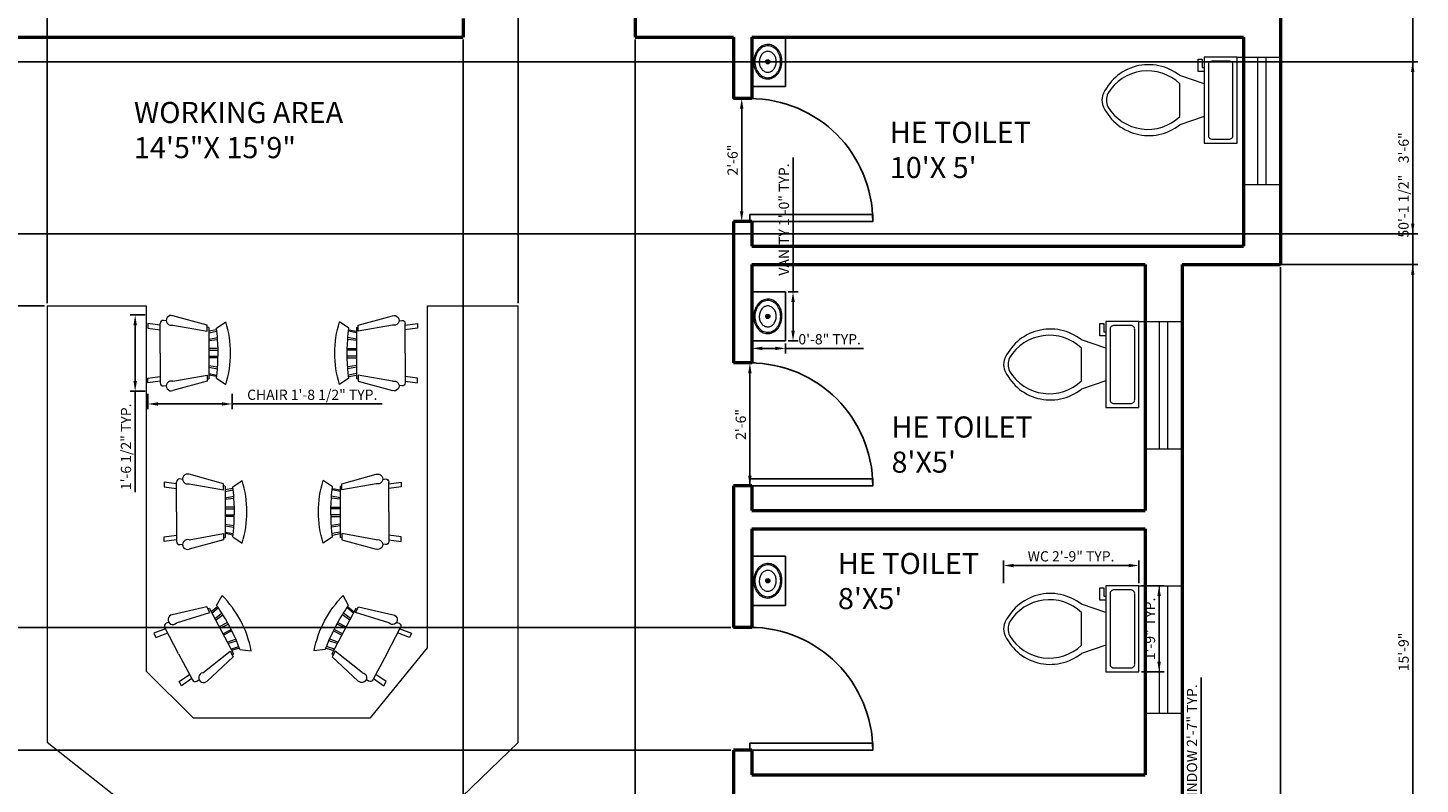
# Model space of a CAD drawing. Units: inches. Extents: x -4852 to -4300, y 4342 to 5059.
# Tile 3 of 4: x -4640 to -4300, y 4580 to 4764. Entities that reach past the tile are written whole.
import ezdxf

# ---------------------------------------------------------------- set-up
doc = ezdxf.new("R2010")
doc.units = ezdxf.units.IN
for name, color, linetype, lineweight in [('A-ANNO-DIMS', 2, 'Continuous', 18), ('A-AREA-IDEN', 7, 'Continuous', 18), ('A-DOOR', 4, 'Continuous', 25), ('A-FLOR-CASE', 9, 'Continuous', 25), ('A-FLOR-FIXT', 9, 'Continuous', 18), ('A-FURN', 8, 'Continuous', 18), ('A-GLAZ', 4, 'Continuous', 18), ('A-WALL', 7, 'Continuous', 50)]:
    doc.layers.add(name, color=color, linetype=linetype, lineweight=lineweight)
doc.styles.get("Standard").update_dxf_attribs({"font": 'arial.ttf'})
doc.dimstyles.new('ISO-25', dxfattribs={"dimtxt": 2.5, "dimasz": 2.5, "dimexe": 1.25, "dimexo": 0.625, "dimtad": 1, "dimdec": 0, "dimlunit": 3, "dimtxsty": 'Standard', "dimcen": 2.5, "dimadec": 0, "dimazin": 0, "dimtfac": 1, "dimtdec": 0, "dimtmove": 0, "dimatfit": 3, "dimfxl": 1, "dimarcsym": 0})

# ---------------------------------------------------------------- blocks, each defined once
blk = doc.blocks.new('*U2')
for p, q in [((0, 0), (0, -100)), ((750, 0), (750, -100))]:
    blk.add_line(p, q)
blk.add_lwpolyline([(0, 0), (0, 750), (43.75, 750), (43.75, 0)], close=True)
blk.add_arc((0, 0), 750, 0, 90)
blk = doc.blocks.new('Toilet - top')
for p, q in [((9.5, -6), (9.5, -2)), ((-10, -8.5), (-8, -8.5)), ((-10, -9.5), (-10, -8.5)), ((-7, -9.5), (-10, -9.5)), ((-8, -8.5), (-8, -8)), ((-7, -8), (-7, -9.5)), ((-4, -8), (-6, -14)), ((4, -8), (6, -14)), ((4, -14), (-4, -14))]:
    blk.add_line(p, q)
blk.add_lwpolyline([(10.5, -8), (10.5, 0), (-10.5, 0), (-10.5, -8)], close=True)
for points in [[(-9.5, -2), (-9.5, -6)], [(8.5, -1), (-8.5, -1)], [(-8.5, -7), (8.5, -7)]]:
    blk.add_lwpolyline(points)
for centre, radius, start, end in [((-8.62, -1.88), 0.884, 81.8699, 188.1301), ((8.62, -1.88), 0.884, 351.8699, 98.1301), ((-8.62, -6.12), 0.884, 171.8699, 278.1301), ((8.62, -6.12), 0.884, 261.8699, 8.1301), ((3.52, -21.58), 12.17, 141.4691, 247.9714), ((4.2, -21.82), 11.33, 136.3677, 238.9468), ((-3.52, -21.58), 12.17, 292.0284, 38.5307), ((-4.2, -21.82), 11.33, 301.053, 43.6321), ((0, -27.88), 4, 245.7318, 294.2682), ((0, -29), 4, 254.8605, 285.1395)]:
    blk.add_arc(centre, radius, start, end)
blk = doc.blocks.new('Sink - Oval top')
for p, q in [((-1, 0), (1, 0)), ((0, 1), (0, -1))]:
    blk.add_line(p, q)
for points in [[(-12.23, 0.39, 0.117634), (-11.46, -3.36, 0.104469), (-8.88, -6.8, 0.090016), (-5.08, -9.07, 0.08192), (-0.32, -10.02, 0.08192), (4.49, -9.38, 0.090016), (8.42, -7.36, 0.104469), (11.22, -4.09, 0.117634), (12.23, -0.39, 0.117634), (11.46, 3.36, 0.104469), (8.88, 6.8, 0.090016), (5.08, 9.07, 0.08192), (0.32, 10.02, 0.08192), (-4.49, 9.38, 0.090016), (-8.42, 7.36, 0.104469), (-11.22, 4.09, 0.117634)], [(-11.29, 0.16, 0.118622), (-10.52, -3.25, 0.104678), (-8.07, -6.36, 0.089562), (-4.54, -8.37, 0.081185), (-0.13, -9.15, 0.081185), (4.3, -8.49, 0.089562), (7.89, -6.58, 0.104678), (10.42, -3.55, 0.118622), (11.29, -0.16, 0.118622), (10.52, 3.25, 0.104678), (8.07, 6.36, 0.089562), (4.54, 8.37, 0.081185), (0.13, 9.15, 0.081185), (-4.3, 8.49, 0.089562), (-7.89, 6.58, 0.104678), (-10.42, 3.55, 0.118622)], [(-7.42, 0.08, 0.118283), (-6.91, -2.17, 0.104607), (-5.29, -4.21, 0.089718), (-2.97, -5.53, 0.081436), (-0.07, -6.04, 0.081436), (2.84, -5.59, 0.089718), (5.2, -4.33, 0.104607), (6.86, -2.32, 0.118283), (7.42, -0.08, 0.118283), (6.91, 2.17, 0.104607), (5.29, 4.21, 0.089718), (2.97, 5.53, 0.081436), (0.07, 6.04, 0.081436), (-2.84, 5.59, 0.089718), (-5.2, 4.33, 0.104607), (-6.86, 2.32, 0.118283)]]:
    blk.add_lwpolyline(points, format="xyb", close=True)
for radius in [1.5, 1]:
    blk.add_circle((0, 0), radius)
blk = doc.blocks.new('Chair - Rocking')
for p, q in [((-8, -4.5), (-10, -1.5)), ((-6.5, -7), (-7.02225, -4.43)), ((-4.5, -7), (-4.96674, -4.19951)), ((-4, -7), (-4.40532, -4.16272)), ((-1.5, -4.05012), (-1.5, -7)), ((-1, -7), (-1, -4.05012)), ((1, -7), (1, -4.04655)), ((1.5, -4.05012), (1.5, -7)), ((4, -7), (4.40187, -4.18694)), ((4.5, -7), (4.96761, -4.19437)), ((6.5, -7), (7, -4.4057)), ((8, -4.5), (10, -1.5)), ((-9, -7.5), (-12, -18.49999)), ((-7, -7.5), (-9, -7.5)), ((-9, -18.49999), (-7, -7.5)), ((-8.23428, -6.99939), (-8.3093, -7.47958)), ((-8.23041, -7), (8.23915, -7)), ((-7.5, -4.5), (-7, -7)), ((7.5, -4.5), (7, -7)), ((7, -7.5), (9, -7.5)), ((9, -18.49999), (7, -7.5)), ((8.31071, -7.48854), (8.23449, -7.00073)), ((9, -7.5), (12, -18.49999)), ((-10.36644, -20.64523), (-10.5, -21.49999)), ((10.5, -21.49999), (10.3575, -20.58798)), ((-9, -22.49999), (-9.5, -26.49999)), ((0, -22.49999), (-9.5, -22.49999)), ((-9.5, -26.49999), (-8, -26.49999)), ((-8, -26.49999), (-7.5, -22.49999)), ((0, -22.49999), (9.5, -22.49999)), ((8, -26.49999), (7.5, -22.49999)), ((9.5, -26.49999), (8, -26.49999)), ((9, -22.49999), (9.5, -26.49999))]:
    blk.add_line(p, q)
for centre, radius, start, end in [((0, -34.08333), 34.08333, 72.93847, 107.0615), ((0, -68.25004), 64.25, 93.92211, 97.15267), ((0, -68.25004), 64.25, 82.84733, 93.92211), ((-10.5, -18.99999), 1.58114, 161.5651, 18.43495), ((-9.5, -21.49999), 1, 180, 270), ((10.5, -18.99999), 1.58114, 161.5651, 18.43495), ((9.5, -21.49999), 1, 270, 0)]:
    blk.add_arc(centre, radius, start, end)
blk = doc.blocks.new('*D12')
at = {"layer": 'A-ANNO-DIMS', "color": 0, "lineweight": -2, "transparency": 16777216}
for p, q in [((-4466.77, 4682.38), (-4462.15, 4682.38)), ((-4463.4, 4679.88), (-4463.4, 4654.88)), ((-4464.52, 4652.38), (-4462.15, 4652.38))]:
    blk.add_line(p, q, dxfattribs=at)
at = {"layer": 'A-ANNO-DIMS', "color": 0, "transparency": 16777216}
for points in [[(-4463.82, 4679.88), (-4462.98, 4679.88), (-4463.4, 4682.38)], [(-4463.82, 4654.88), (-4462.98, 4654.88), (-4463.4, 4652.38)]]:
    blk.add_solid(points, dxfattribs=at)
at = {"layer": 'Defpoints', "color": 0, "transparency": 16777216}
for p in [(-4467.4, 4682.38), (-4465.15, 4652.38), (-4463.4, 4652.38)]:
    blk.add_point(p, dxfattribs=at)
at = {"layer": 'A-ANNO-DIMS', "color": 0, "transparency": 16777216, "insert": (-4465.3, 4667.38), "char_height": 2.5, "attachment_point": 5, "rotation": 90}
blk.add_mtext('2\'-6"', dxfattribs=at)
blk = doc.blocks.new('*D13')
at = {"layer": 'A-ANNO-DIMS', "color": 0, "lineweight": -2, "transparency": 16777216}
for p, q in [((-4466.77, 4746.88), (-4464.15, 4746.88)), ((-4465.4, 4744.38), (-4465.4, 4719.38)), ((-4466.02, 4716.88), (-4466.65, 4716.88))]:
    blk.add_line(p, q, dxfattribs=at)
at = {"layer": 'A-ANNO-DIMS', "color": 0, "transparency": 16777216}
for points in [[(-4465.82, 4744.38), (-4464.98, 4744.38), (-4465.4, 4746.88)], [(-4465.82, 4719.38), (-4464.98, 4719.38), (-4465.4, 4716.88)]]:
    blk.add_solid(points, dxfattribs=at)
at = {"layer": 'Defpoints', "color": 0, "transparency": 16777216}
for p in [(-4467.4, 4746.88), (-4465.4, 4716.88), (-4465.4, 4716.88)]:
    blk.add_point(p, dxfattribs=at)
at = {"layer": 'A-ANNO-DIMS', "color": 0, "transparency": 16777216, "insert": (-4467.3, 4731.88), "char_height": 2.5, "attachment_point": 5, "rotation": 90}
blk.add_mtext('2\'-6"', dxfattribs=at)
blk = doc.blocks.new('VANITY-COMPACT')
for p, q in [((8.23, 12.02), (0, 12.02)), ((8.23, 0), (8.23, 12.02)), ((0, 0), (8.23, 0))]:
    blk.add_line(p, q)
blk = doc.blocks.new('WIN-RESTROOM')
for p, q in [((0, 31.05), (10.57, 31.05)), ((5.07, 0), (5.07, 31.05)), ((7.07, 0), (7.07, 31.05)), ((1.57, 0), (10.57, 0))]:
    blk.add_line(p, q)
blk = doc.blocks.new('*D23')
at = {"layer": 'A-ANNO-DIMS', "color": 0, "lineweight": -2, "transparency": 16777216}
for p, q in [((-4610.37, 4674.84), (-4610.37, 4671.12)), ((-4589.8, 4674.84), (-4589.8, 4671.12)), ((-4607.87, 4672.37), (-4592.3, 4672.37)), ((-4589.8, 4672.37), (-4553.17, 4672.37))]:
    blk.add_line(p, q, dxfattribs=at)
at = {"layer": 'A-ANNO-DIMS', "color": 0, "transparency": 16777216}
for points in [[(-4607.87, 4672.79), (-4607.87, 4671.96), (-4610.37, 4672.37)], [(-4592.3, 4672.79), (-4592.3, 4671.96), (-4589.8, 4672.37)]]:
    blk.add_solid(points, dxfattribs=at)
at = {"layer": 'Defpoints', "color": 0, "transparency": 16777216}
for p in [(-4610.37, 4675.46), (-4589.8, 4675.46), (-4589.8, 4672.37)]:
    blk.add_point(p, dxfattribs=at)
at = {"layer": 'A-ANNO-DIMS', "color": 0, "transparency": 16777216, "insert": (-4570.23, 4674.29), "char_height": 2.5, "attachment_point": 5}
blk.add_mtext('CHAIR 1\'-8 1/2" TYP.', dxfattribs=at)
blk = doc.blocks.new('*D24')
at = {"layer": 'A-ANNO-DIMS', "color": 0, "lineweight": -2, "transparency": 16777216}
for p, q in [((-4611, 4694.08), (-4614.71, 4694.08)), ((-4613.46, 4691.58), (-4613.46, 4677.96)), ((-4611, 4675.46), (-4614.71, 4675.46)), ((-4613.46, 4675.46), (-4613.46, 4650.88))]:
    blk.add_line(p, q, dxfattribs=at)
at = {"layer": 'A-ANNO-DIMS', "color": 0, "transparency": 16777216}
for points in [[(-4613.88, 4691.58), (-4613.04, 4691.58), (-4613.46, 4694.08)], [(-4613.88, 4677.96), (-4613.04, 4677.96), (-4613.46, 4675.46)]]:
    blk.add_solid(points, dxfattribs=at)
at = {"layer": 'Defpoints', "color": 0, "transparency": 16777216}
for p in [(-4610.37, 4694.08), (-4613.46, 4675.46), (-4610.37, 4675.46)]:
    blk.add_point(p, dxfattribs=at)
at = {"layer": 'A-ANNO-DIMS', "color": 0, "transparency": 16777216, "insert": (-4615.38, 4661.92), "char_height": 2.5, "attachment_point": 5, "rotation": 90}
blk.add_mtext('1\'-6 1/2" TYP.', dxfattribs=at)
blk = doc.blocks.new('*D27')
at = {"layer": 'A-ANNO-DIMS', "color": 0, "lineweight": -2, "transparency": 16777216}
for p, q in [((-4401.51, 4628.63), (-4401.51, 4634.21)), ((-4399.01, 4632.96), (-4370.97, 4632.96)), ((-4368.47, 4628.63), (-4368.47, 4634.21))]:
    blk.add_line(p, q, dxfattribs=at)
at = {"layer": 'A-ANNO-DIMS', "color": 0, "transparency": 16777216}
for points in [[(-4399.01, 4633.38), (-4399.01, 4632.54), (-4401.51, 4632.96)], [(-4370.97, 4633.38), (-4370.97, 4632.54), (-4368.47, 4632.96)]]:
    blk.add_solid(points, dxfattribs=at)
at = {"layer": 'Defpoints', "color": 0, "transparency": 16777216}
for p in [(-4368.47, 4632.96), (-4401.51, 4628), (-4368.47, 4628)]:
    blk.add_point(p, dxfattribs=at)
at = {"layer": 'A-ANNO-DIMS', "color": 0, "transparency": 16777216, "insert": (-4384.99, 4634.88), "char_height": 2.5, "attachment_point": 5}
blk.add_mtext('WC 2\'-9" TYP.', dxfattribs=at)
blk = doc.blocks.new('*D28')
at = {"layer": 'A-ANNO-DIMS', "color": 0, "lineweight": -2, "transparency": 16777216}
for p, q in [((-4367.84, 4628), (-4362.26, 4628)), ((-4363.51, 4625.5), (-4363.51, 4609.5)), ((-4367.84, 4607), (-4362.26, 4607))]:
    blk.add_line(p, q, dxfattribs=at)
at = {"layer": 'A-ANNO-DIMS', "color": 0, "transparency": 16777216}
for points in [[(-4363.93, 4625.5), (-4363.09, 4625.5), (-4363.51, 4628)], [(-4363.93, 4609.5), (-4363.09, 4609.5), (-4363.51, 4607)]]:
    blk.add_solid(points, dxfattribs=at)
at = {"layer": 'Defpoints', "color": 0, "transparency": 16777216}
for p in [(-4368.47, 4628), (-4368.47, 4607), (-4363.51, 4607)]:
    blk.add_point(p, dxfattribs=at)
at = {"layer": 'A-ANNO-DIMS', "color": 0, "transparency": 16777216, "insert": (-4365.41, 4617.5), "char_height": 2.5, "attachment_point": 5, "rotation": 90}
blk.add_mtext('1\'-9" TYP.', dxfattribs=at)
blk = doc.blocks.new('*D33')
at = {"layer": 'A-ANNO-DIMS', "color": 0, "lineweight": -2, "transparency": 16777216}
for p, q in [((-4452.87, 4699.76), (-4452.87, 4732.47)), ((-4454.04, 4699.76), (-4451.62, 4699.76)), ((-4452.87, 4690.24), (-4452.87, 4697.26)), ((-4454.04, 4687.74), (-4451.62, 4687.74))]:
    blk.add_line(p, q, dxfattribs=at)
at = {"layer": 'A-ANNO-DIMS', "color": 0, "transparency": 16777216}
for points in [[(-4453.28, 4697.26), (-4452.45, 4697.26), (-4452.87, 4699.76)], [(-4453.28, 4690.24), (-4452.45, 4690.24), (-4452.87, 4687.74)]]:
    blk.add_solid(points, dxfattribs=at)
at = {"layer": 'Defpoints', "color": 0, "transparency": 16777216}
for p in [(-4454.67, 4699.76), (-4452.87, 4699.76), (-4454.67, 4687.74)]:
    blk.add_point(p, dxfattribs=at)
at = {"layer": 'A-ANNO-DIMS', "color": 0, "transparency": 16777216, "insert": (-4454.77, 4717.37), "char_height": 2.5, "attachment_point": 5, "rotation": 90}
blk.add_mtext('VANITY 1\'-0" TYP.', dxfattribs=at)
blk = doc.blocks.new('*D34')
at = {"layer": 'A-ANNO-DIMS', "color": 0, "lineweight": -2, "transparency": 16777216}
for p, q in [((-4462.9, 4687.12), (-4462.9, 4684.69)), ((-4454.67, 4687.12), (-4454.67, 4684.69)), ((-4460.4, 4685.94), (-4457.17, 4685.94)), ((-4454.67, 4685.94), (-4435.68, 4685.94))]:
    blk.add_line(p, q, dxfattribs=at)
at = {"layer": 'A-ANNO-DIMS', "color": 0, "transparency": 16777216}
for points in [[(-4460.4, 4686.35), (-4460.4, 4685.52), (-4462.9, 4685.94)], [(-4457.17, 4686.35), (-4457.17, 4685.52), (-4454.67, 4685.94)]]:
    blk.add_solid(points, dxfattribs=at)
at = {"layer": 'Defpoints', "color": 0, "transparency": 16777216}
for p in [(-4462.9, 4687.74), (-4454.67, 4687.74), (-4454.67, 4685.94)]:
    blk.add_point(p, dxfattribs=at)
at = {"layer": 'A-ANNO-DIMS', "color": 0, "transparency": 16777216, "insert": (-4443.93, 4687.84), "char_height": 2.5, "attachment_point": 5}
blk.add_mtext('0\'-8" TYP.', dxfattribs=at)
blk = doc.blocks.new('*D35')
at = {"layer": 'A-ANNO-DIMS', "color": 0, "lineweight": -2, "transparency": 16777216}
for p, q in [((-4353.24, 4563.5), (-4353.24, 4605.68)), ((-4357.27, 4563.5), (-4351.99, 4563.5)), ((-4353.24, 4534.95), (-4353.24, 4561)), ((-4357.27, 4532.45), (-4351.99, 4532.45))]:
    blk.add_line(p, q, dxfattribs=at)
at = {"layer": 'A-ANNO-DIMS', "color": 0, "transparency": 16777216}
for points in [[(-4353.66, 4561), (-4352.83, 4561), (-4353.24, 4563.5)], [(-4353.66, 4534.95), (-4352.83, 4534.95), (-4353.24, 4532.45)]]:
    blk.add_solid(points, dxfattribs=at)
at = {"layer": 'Defpoints', "color": 0, "transparency": 16777216}
for p in [(-4357.9, 4563.5), (-4353.24, 4563.5), (-4357.9, 4532.45)]:
    blk.add_point(p, dxfattribs=at)
at = {"layer": 'A-ANNO-DIMS', "color": 0, "transparency": 16777216, "insert": (-4355.16, 4585.84), "char_height": 2.5, "attachment_point": 5, "rotation": 90}
blk.add_mtext('WC WINDOW 2\'-7" TYP.', dxfattribs=at)
blk = doc.blocks.new('*D40')
at = {"layer": 'A-ANNO-DIMS', "color": 0, "lineweight": -2, "transparency": 16777216}
for p, q in [((-4333.27, 5021.38), (-4300.34, 5021.38)), ((-4301.59, 4422.38), (-4301.59, 5018.88)), ((-4333.27, 4419.88), (-4300.34, 4419.88))]:
    blk.add_line(p, q, dxfattribs=at)
at = {"layer": 'A-ANNO-DIMS', "color": 0, "transparency": 16777216}
for points in [[(-4302.01, 5018.88), (-4301.17, 5018.88), (-4301.59, 5021.38)], [(-4302.01, 4422.38), (-4301.17, 4422.38), (-4301.59, 4419.88)]]:
    blk.add_solid(points, dxfattribs=at)
at = {"layer": 'Defpoints', "color": 0, "transparency": 16777216}
for p in [(-4333.9, 5021.38), (-4301.59, 5021.38), (-4333.9, 4419.88)]:
    blk.add_point(p, dxfattribs=at)
at = {"layer": 'A-ANNO-DIMS', "color": 0, "transparency": 16777216, "insert": (-4303.51, 4720.63), "char_height": 2.5, "attachment_point": 5, "rotation": 90}
blk.add_mtext('50\'-1 1/2"', dxfattribs=at)
blk = doc.blocks.new('*D43')
at = {"layer": 'A-ANNO-DIMS', "color": 0, "lineweight": -2, "transparency": 16777216}
for p, q in [((-4357.9, 4705.75), (-4357.9, 4342.18)), ((-4333.9, 4705.75), (-4333.9, 4342.18)), ((-4355.4, 4343.43), (-4336.4, 4343.43))]:
    blk.add_line(p, q, dxfattribs=at)
at = {"layer": 'A-ANNO-DIMS', "color": 0, "transparency": 16777216}
for points in [[(-4355.4, 4343.85), (-4355.4, 4343.01), (-4357.9, 4343.43)], [(-4336.4, 4343.85), (-4336.4, 4343.01), (-4333.9, 4343.43)]]:
    blk.add_solid(points, dxfattribs=at)
at = {"layer": 'Defpoints', "color": 0, "transparency": 16777216}
for p in [(-4357.9, 4706.38), (-4333.9, 4706.38), (-4333.9, 4343.43)]:
    blk.add_point(p, dxfattribs=at)
at = {"layer": 'A-ANNO-DIMS', "color": 0, "transparency": 16777216, "insert": (-4345.9, 4345.33), "char_height": 2.5, "attachment_point": 5}
blk.add_mtext('2\'-0"', dxfattribs=at)
blk = doc.blocks.new('*D44')
at = {"layer": 'A-ANNO-DIMS', "color": 0, "lineweight": -2, "transparency": 16777216}
for p, q in [((-4357.27, 4706.38), (-4300.34, 4706.38)), ((-4301.59, 4519.88), (-4301.59, 4703.88)), ((-4357.27, 4517.38), (-4300.34, 4517.38))]:
    blk.add_line(p, q, dxfattribs=at)
at = {"layer": 'A-ANNO-DIMS', "color": 0, "transparency": 16777216}
for points in [[(-4302.01, 4703.88), (-4301.17, 4703.88), (-4301.59, 4706.38)], [(-4302.01, 4519.88), (-4301.17, 4519.88), (-4301.59, 4517.38)]]:
    blk.add_solid(points, dxfattribs=at)
at = {"layer": 'Defpoints', "color": 0, "transparency": 16777216}
for p in [(-4357.9, 4706.38), (-4301.59, 4706.38), (-4357.9, 4517.38)]:
    blk.add_point(p, dxfattribs=at)
at = {"layer": 'A-ANNO-DIMS', "color": 0, "transparency": 16777216, "insert": (-4303.49, 4611.88), "char_height": 2.5, "attachment_point": 5, "rotation": 90}
blk.add_mtext('15\'-9"', dxfattribs=at)
blk = doc.blocks.new('*D46')
at = {"layer": 'A-ANNO-DIMS', "color": 0, "lineweight": -2, "transparency": 16777216}
for p, q in [((-4679.77, 4755.88), (-4300.34, 4755.88)), ((-4301.59, 4716.38), (-4301.59, 4753.38)), ((-4679.77, 4713.88), (-4300.34, 4713.88))]:
    blk.add_line(p, q, dxfattribs=at)
at = {"layer": 'A-ANNO-DIMS', "color": 0, "transparency": 16777216}
for points in [[(-4302.01, 4753.38), (-4301.17, 4753.38), (-4301.59, 4755.88)], [(-4302.01, 4716.38), (-4301.17, 4716.38), (-4301.59, 4713.88)]]:
    blk.add_solid(points, dxfattribs=at)
at = {"layer": 'Defpoints', "color": 0, "transparency": 16777216}
for p in [(-4680.4, 4755.88), (-4301.59, 4755.88), (-4680.4, 4713.88)]:
    blk.add_point(p, dxfattribs=at)
at = {"layer": 'A-ANNO-DIMS', "color": 0, "transparency": 16777216, "insert": (-4303.49, 4734.88), "char_height": 2.5, "attachment_point": 5, "rotation": 90}
blk.add_mtext('3\'-6"', dxfattribs=at)
blk = doc.blocks.new('*D48')
at = {"layer": 'A-ANNO-DIMS', "color": 0, "lineweight": -2, "transparency": 16777216}
for p, q in [((-4468.02, 4617.88), (-4847.46, 4617.88)), ((-4846.21, 4590.38), (-4846.21, 4615.38)), ((-4468.02, 4587.88), (-4847.46, 4587.88))]:
    blk.add_line(p, q, dxfattribs=at)
at = {"layer": 'A-ANNO-DIMS', "color": 0, "transparency": 16777216}
for points in [[(-4846.63, 4615.38), (-4845.79, 4615.38), (-4846.21, 4617.88)], [(-4846.63, 4590.38), (-4845.79, 4590.38), (-4846.21, 4587.88)]]:
    blk.add_solid(points, dxfattribs=at)
at = {"layer": 'Defpoints', "color": 0, "transparency": 16777216}
for p in [(-4846.21, 4617.88), (-4467.4, 4617.88), (-4467.4, 4587.88)]:
    blk.add_point(p, dxfattribs=at)
at = {"layer": 'A-ANNO-DIMS', "color": 0, "transparency": 16777216, "insert": (-4848.11, 4602.88), "char_height": 2.5, "attachment_point": 5, "rotation": 90}
blk.add_mtext('2\'-6"', dxfattribs=at)
blk = doc.blocks.new('*D59')
at = {"layer": 'A-ANNO-DIMS', "color": 0, "lineweight": -2, "transparency": 16777216}
for p, q in [((-4533.4, 4761.25), (-4533.4, 4342.18)), ((-4491.4, 4761.25), (-4491.4, 4342.18)), ((-4530.9, 4343.43), (-4493.9, 4343.43))]:
    blk.add_line(p, q, dxfattribs=at)
at = {"layer": 'A-ANNO-DIMS', "color": 0, "transparency": 16777216}
for points in [[(-4530.9, 4343.85), (-4530.9, 4343.01), (-4533.4, 4343.43)], [(-4493.9, 4343.85), (-4493.9, 4343.01), (-4491.4, 4343.43)]]:
    blk.add_solid(points, dxfattribs=at)
at = {"layer": 'Defpoints', "color": 0, "transparency": 16777216}
for p in [(-4533.4, 4761.88), (-4491.4, 4761.88), (-4491.4, 4343.43)]:
    blk.add_point(p, dxfattribs=at)
at = {"layer": 'A-ANNO-DIMS', "color": 0, "transparency": 16777216, "insert": (-4512.4, 4345.33), "char_height": 2.5, "attachment_point": 5}
blk.add_mtext('3\'-6"', dxfattribs=at)
blk = doc.blocks.new('*D60')
at = {"layer": 'A-ANNO-DIMS', "color": 0, "lineweight": -2, "transparency": 16777216}
for p, q in [((-4634.93, 4696.96), (-4634.93, 5054.94)), ((-4519.98, 4696.96), (-4519.98, 5054.94)), ((-4632.43, 5053.69), (-4522.48, 5053.69))]:
    blk.add_line(p, q, dxfattribs=at)
at = {"layer": 'A-ANNO-DIMS', "color": 0, "transparency": 16777216}
for points in [[(-4632.43, 5054.11), (-4632.43, 5053.27), (-4634.93, 5053.69)], [(-4522.48, 5054.11), (-4522.48, 5053.27), (-4519.98, 5053.69)]]:
    blk.add_solid(points, dxfattribs=at)
at = {"layer": 'Defpoints', "color": 0, "transparency": 16777216}
for p in [(-4519.98, 5053.69), (-4634.93, 4696.34), (-4519.98, 4696.34)]:
    blk.add_point(p, dxfattribs=at)
at = {"layer": 'A-ANNO-DIMS', "color": 0, "transparency": 16777216, "insert": (-4577.45, 5055.59), "char_height": 2.5, "attachment_point": 5}
blk.add_mtext('9\'-7"', dxfattribs=at)
blk = doc.blocks.new('*D61')
at = {"layer": 'A-ANNO-DIMS', "color": 0, "lineweight": -2, "transparency": 16777216}
for p, q in [((-4635.56, 4696.34), (-4847.46, 4696.34)), ((-4846.21, 4693.84), (-4846.21, 4570.1)), ((-4607.33, 4567.6), (-4847.46, 4567.6))]:
    blk.add_line(p, q, dxfattribs=at)
at = {"layer": 'A-ANNO-DIMS', "color": 0, "transparency": 16777216}
for points in [[(-4846.63, 4693.84), (-4845.79, 4693.84), (-4846.21, 4696.34)], [(-4846.63, 4570.1), (-4845.79, 4570.1), (-4846.21, 4567.6)]]:
    blk.add_solid(points, dxfattribs=at)
at = {"layer": 'Defpoints', "color": 0, "transparency": 16777216}
for p in [(-4634.93, 4696.34), (-4846.21, 4567.6), (-4606.71, 4567.6)]:
    blk.add_point(p, dxfattribs=at)
at = {"layer": 'A-ANNO-DIMS', "color": 0, "transparency": 16777216, "insert": (-4848.13, 4631.97), "char_height": 2.5, "attachment_point": 5, "rotation": 90}
blk.add_mtext('10\'-8 1/2"', dxfattribs=at)

msp = doc.modelspace()

# ---------------------------------------------------------------- linework, layer by layer
at = {"layer": 'A-FURN'}
for p, q in [((-4634.93, 4696.34), (-4634.93, 4589.86)), ((-4634.93, 4696.34), (-4610.79, 4696.34)), ((-4610.79, 4696.34), (-4610.79, 4607.17)), ((-4542.13, 4612.91), (-4542.13, 4696.34)), ((-4542.13, 4696.34), (-4519.98, 4696.34)), ((-4519.98, 4589.79), (-4519.98, 4696.34)), ((-4556.04, 4595.84), (-4542.13, 4612.91)), ((-4610.79, 4607.17), (-4599.29, 4595.84)), ((-4599.29, 4595.84), (-4556.04, 4595.84)), ((-4634.93, 4589.86), (-4606.71, 4567.6)), ((-4543.07, 4567.6), (-4519.98, 4589.79))]:
    msp.add_line(p, q, dxfattribs=at)
at = {"layer": 'A-WALL'}
for p, q in [((-4333.9, 5021.38), (-4333.9, 4706.38)), ((-4491.4, 4772.38), (-4491.4, 4761.88)), ((-4533.4, 4766.38), (-4533.4, 4761.88)), ((-4680.4, 4761.88), (-4533.4, 4761.88)), ((-4491.4, 4761.88), (-4467.4, 4761.88)), ((-4486.9, 4761.88), (-4467.4, 4761.88)), ((-4467.4, 4761.88), (-4467.4, 4746.88)), ((-4462.9, 4761.88), (-4462.9, 4746.88)), ((-4462.9, 4761.88), (-4342.9, 4761.88)), ((-4462.9, 4761.88), (-4342.9, 4761.88)), ((-4342.9, 4761.88), (-4342.9, 4710.88)), ((-4462.9, 4746.88), (-4467.4, 4746.88)), ((-4462.9, 4716.88), (-4467.4, 4716.88)), ((-4467.4, 4716.88), (-4467.4, 4682.38)), ((-4462.9, 4716.88), (-4462.9, 4710.88)), ((-4462.9, 4710.88), (-4342.9, 4710.88)), ((-4462.9, 4706.38), (-4366.9, 4706.38)), ((-4462.9, 4706.38), (-4462.9, 4682.38)), ((-4366.9, 4706.38), (-4366.9, 4646.38)), ((-4357.9, 4706.38), (-4357.9, 4517.38)), ((-4357.9, 4706.38), (-4333.9, 4706.38)), ((-4462.9, 4682.38), (-4467.4, 4682.38)), ((-4462.9, 4652.38), (-4467.4, 4652.38)), ((-4467.4, 4652.38), (-4467.4, 4617.88)), ((-4462.9, 4652.38), (-4462.9, 4646.38)), ((-4462.9, 4646.38), (-4366.9, 4646.38)), ((-4462.9, 4641.88), (-4366.9, 4641.88)), ((-4462.9, 4641.88), (-4462.9, 4617.88)), ((-4366.9, 4641.88), (-4366.9, 4581.88)), ((-4462.9, 4617.88), (-4467.4, 4617.88)), ((-4462.9, 4587.88), (-4467.4, 4587.88)), ((-4467.4, 4587.88), (-4467.4, 4553.38)), ((-4462.9, 4587.88), (-4462.9, 4581.88)), ((-4462.9, 4581.88), (-4366.9, 4581.88))]:
    msp.add_line(p, q, dxfattribs=at)

# ---------------------------------------------------------------- block references
at = {"layer": 'A-DOOR', "xscale": -0.0399999999999999, "yscale": 0.0399999999999999, "zscale": 0.0399999999999999, "rotation": 270}
for p in [(-4463.4, 4716.88), (-4463.4, 4652.38), (-4463.4, 4587.88)]:
    msp.add_blockref('*U2', p, dxfattribs=at)
at = {"layer": 'A-FLOR-CASE'}
for p in [(-4462.9, 4749.85), (-4462.9, 4687.74), (-4462.9, 4623.24)]:
    msp.add_blockref('VANITY-COMPACT', p, dxfattribs=at)
at = {"layer": 'A-FLOR-FIXT', "xscale": 0.343836899682101, "yscale": 0.343836899682101, "zscale": 0.343836899682101, "rotation": 270}
for p in [(-4459.03, 4755.86), (-4459.03, 4693.74), (-4459.03, 4629.24)]:
    msp.add_blockref('Sink - Oval top', p, dxfattribs=at)
at = {"layer": 'A-FLOR-FIXT', "rotation": 270}
for p in [(-4344.47, 4746.5), (-4368.47, 4682), (-4368.47, 4617.5)]:
    msp.add_blockref('Toilet - top', p, dxfattribs=at)
at = {"layer": 'A-FURN', "yscale": 0.7621443616854127, "zscale": 0.7621443616854127}
for p, xscale, rotation in [((-4590.18, 4684.77), 0.7621443616854127, 270), ((-4564.74, 4684.77), -0.7621443616854127, 90), ((-4586.19, 4646.07), 0.7621443616854127, 270), ((-4568.72, 4646.07), -0.7621443616854127, 90), ((-4587.69, 4619.46), 0.7621443616854127, 297.842284233736), ((-4567.23, 4619.46), -0.7621443616854127, 62.15771576626402)]:
    msp.add_blockref('Chair - Rocking', p, dxfattribs=dict(at, xscale=xscale, rotation=rotation))
at = {"layer": 'A-GLAZ'}
for p in [(-4344.47, 4725.95), (-4368.47, 4661.45), (-4368.47, 4596.95)]:
    msp.add_blockref('WIN-RESTROOM', p, dxfattribs=at)

# ---------------------------------------------------------------- texts
at = {"layer": 'A-AREA-IDEN'}
for s, height, p in [('WORKING AREA', 5.1489, (-4613.76, 4740.91)), ('HE TOILET', 5.149, (-4429.25, 4736.06)), ('14\'5"X 15\'9"', 5.1489, (-4613.76, 4732.34)), ("10'X 5'", 5.149, (-4429.25, 4727.49)), ('HE TOILET', 5.149, (-4428.83, 4664.18)), ("8'X5'", 5.149, (-4428.83, 4655.61)), ('HE TOILET', 5.149, (-4441.91, 4630.88)), ("8'X5'", 5.149, (-4441.91, 4622.32))]:
    msp.add_text(s, height=height, dxfattribs=at).set_placement(p)

# ---------------------------------------------------------------- dimensions: what is measured, and where the dimension line sits
at = {"layer": 'A-ANNO-DIMS'}
for base, p1, p2, picture, middle in [((-4519.9791, 5053.6893), (-4634.9301, 4696.3372), (-4519.9791, 4696.3372), '*D60', (-4577.4546, 5055.5907)), ((-4491.4, 4343.43), (-4533.4, 4761.88), (-4491.4, 4761.88), '*D59', (-4512.4, 4345.33)), ((-4333.9, 4343.43), (-4357.9, 4706.38), (-4333.9, 4706.38), '*D43', (-4345.9, 4345.33))]:
    dim = msp.add_linear_dim(base=base, p1=p1, p2=p2, dimstyle='ISO-25', override={"dimdec": 1, "dimlfac": 1, "dimrnd": 0, "dimzin": 1, "dimdsep": 46, "dimlunit": 4, "dimfrac": 2}, dxfattribs=at)
    dim.commit()
    dim.dimension.update_dxf_attribs({"geometry": picture, "text_midpoint": middle})
for base, p1, p2, override, picture, middle in [((-4301.59, 5021.38), (-4333.9, 4419.88), (-4333.9, 5021.38), {"dimdec": 1, "dimlfac": 1, "dimrnd": 0, "dimzin": 1, "dimdsep": 46, "dimlunit": 4, "dimfrac": 2}, '*D40', (-4303.51, 4720.63)), ((-4301.59, 4755.88), (-4680.4, 4713.88), (-4680.4, 4755.88), {"dimdec": 1, "dimlfac": 1, "dimrnd": 0, "dimzin": 1, "dimdsep": 46, "dimlunit": 4, "dimfrac": 2}, '*D46', (-4303.49, 4734.88)), ((-4465.4, 4716.88), (-4467.4, 4746.88), (-4465.4, 4716.88), {"dimclrd": 0, "dimclre": 0, "dimclrt": 0}, '*D13', (-4467.3, 4731.88)), ((-4301.59, 4706.38), (-4357.9, 4517.38), (-4357.9, 4706.38), {"dimdec": 1, "dimlfac": 1, "dimrnd": 0, "dimzin": 1, "dimdsep": 46, "dimlunit": 4, "dimfrac": 2}, '*D44', (-4303.49, 4611.88)), ((-4846.21, 4567.6), (-4634.93, 4696.34), (-4606.71, 4567.6), {"dimdec": 1, "dimlfac": 1, "dimrnd": 0, "dimzin": 1, "dimdsep": 46, "dimlunit": 4, "dimfrac": 2}, '*D61', (-4848.13, 4631.97)), ((-4463.4, 4652.38), (-4467.4, 4682.38), (-4465.15, 4652.38), {"dimclrd": 0, "dimclre": 0, "dimclrt": 0}, '*D12', (-4465.3, 4667.38)), ((-4846.21, 4617.88), (-4467.4, 4587.88), (-4467.4, 4617.88), {"dimdec": 1, "dimlfac": 1, "dimrnd": 0, "dimzin": 1, "dimdsep": 46, "dimlunit": 4, "dimfrac": 2}, '*D48', (-4848.11, 4602.88))]:
    dim = msp.add_linear_dim(base=base, p1=p1, p2=p2, angle=90, dimstyle='ISO-25', override=override, dxfattribs=at)
    dim.commit()
    dim.dimension.update_dxf_attribs({"geometry": picture, "text_midpoint": middle})
for base, p1, p2, angle, text, picture, middle in [((-4452.87, 4699.76), (-4454.67, 4687.74), (-4454.67, 4699.76), 90, 'VANITY <> TYP.', '*D33', (-4454.77, 4717.37)), ((-4613.46, 4675.46), (-4610.37, 4694.08), (-4610.37, 4675.46), 270, '<> TYP.', '*D24', (-4615.38, 4661.92)), ((-4363.51, 4607), (-4368.47, 4628), (-4368.47, 4607), 270, '<> TYP.', '*D28', (-4365.41, 4617.5)), ((-4353.242, 4563.5016), (-4357.8994, 4532.4528), (-4357.8994, 4563.5016), 90, 'WC WINDOW <> TYP.', '*D35', (-4355.1605, 4585.8387))]:
    dim = msp.add_linear_dim(base=base, p1=p1, p2=p2, angle=angle, text=text, dimstyle='ISO-25', override={"dimdec": 1, "dimlfac": 1, "dimrnd": 0, "dimzin": 1, "dimdsep": 46, "dimlunit": 4, "dimfrac": 2}, dxfattribs=at)
    dim.commit()
    dim.dimension.update_dxf_attribs({"geometry": picture, "text_midpoint": middle})
for base, p1, p2, text, picture, middle in [((-4454.67, 4685.94), (-4462.9, 4687.74), (-4454.67, 4687.74), '<> TYP.', '*D34', (-4443.93, 4687.84)), ((-4589.8, 4672.37), (-4610.37, 4675.46), (-4589.8, 4675.46), 'CHAIR <> TYP.', '*D23', (-4570.23, 4674.29)), ((-4368.47, 4632.96), (-4401.51, 4628), (-4368.47, 4628), 'WC <> TYP.', '*D27', (-4384.99, 4634.88))]:
    dim = msp.add_linear_dim(base=base, p1=p1, p2=p2, text=text, dimstyle='ISO-25', override={"dimdec": 1, "dimlfac": 1, "dimrnd": 0, "dimzin": 1, "dimdsep": 46, "dimlunit": 4, "dimfrac": 2}, dxfattribs=at)
    dim.commit()
    dim.dimension.update_dxf_attribs({"geometry": picture, "text_midpoint": middle})

doc.saveas('drawing.dxf')
